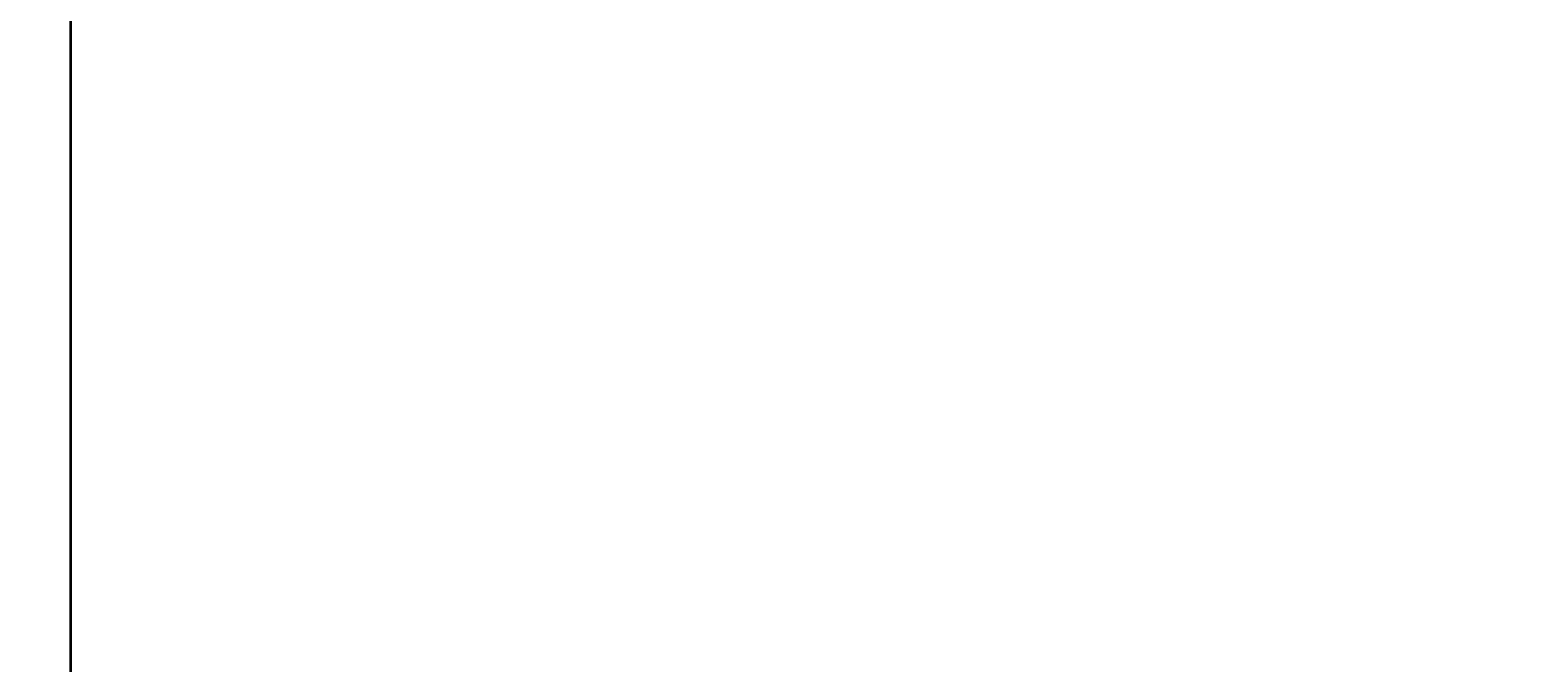
# Model space of a CAD drawing. Units: inches. Extents: x 2163 to 2982, y 1024 to 2288.
# Tile 12 of 22: x 2448 to 2532, y 1885 to 1920. Entities that reach past the tile are written whole.
import ezdxf

# ---------------------------------------------------------------- set-up
doc = ezdxf.new("R2010")
doc.units = ezdxf.units.IN
doc.layers.add('A-ANNO-DIMS', color=2, linetype='Continuous', lineweight=18)
doc.layers.add('A-WALL', color=7, linetype='Continuous', lineweight=35)
doc.styles.get("Standard").update_dxf_attribs({"font": 'arial.ttf'})
doc.dimstyles.get("Standard").update_dxf_attribs({"dimtxt": 0.18, "dimasz": 0.18, "dimexe": 0.18, "dimexo": 0.0625, "dimgap": 0.09, "dimtad": 0, "dimtih": 1, "dimtoh": 1, "dimdec": 4, "dimzin": 0, "dimdsep": 46, "dimtxsty": 'Standard', "dimcen": 0.09, "dimadec": 0, "dimazin": 0, "dimtfac": 1, "dimtdec": 4, "dimtofl": 0, "dimtmove": 0, "dimatfit": 3, "dimfxl": 1, "dimtolj": 1, "dimtzin": 0, "dimarcsym": 0})

# ---------------------------------------------------------------- blocks, each defined once
blk = doc.blocks.new('*D29')
at = {"layer": 'A-ANNO-DIMS', "color": 0, "lineweight": -2, "transparency": 16777216}
for p, q in [((2285.339, 1738.831), (2285.339, 2288.099)), ((2285.519, 2287.919), (2576.051, 2287.919)), ((2867.159, 2287.919), (2576.627, 2287.919)), ((2867.339, 2229.331), (2867.339, 2288.099))]:
    blk.add_line(p, q, dxfattribs=at)
at = {"layer": 'A-ANNO-DIMS', "color": 0, "transparency": 16777216}
for points in [[(2285.519, 2287.949), (2285.519, 2287.889), (2285.339, 2287.919)], [(2867.159, 2287.949), (2867.159, 2287.889), (2867.339, 2287.919)]]:
    blk.add_solid(points, dxfattribs=at)
at = {"layer": 'Defpoints', "color": 0, "transparency": 16777216}
for p in [(2867.339, 2287.919), (2867.339, 2229.269), (2285.339, 1738.769)]:
    blk.add_point(p, dxfattribs=at)
at = {"layer": 'A-ANNO-DIMS', "color": 0, "transparency": 16777216, "insert": (2576.339, 2287.919), "char_height": 0.18, "attachment_point": 5}
blk.add_mtext('\\A1;582', dxfattribs=at)

msp = doc.modelspace()

# ---------------------------------------------------------------- linework, layer by layer
at = {"layer": 'A-WALL'}
msp.add_line((2450.3389, 1963.7688), (2450.3389, 1879.973), dxfattribs=at)

# ---------------------------------------------------------------- dimensions: what is measured, and where the dimension line sits
at = {"layer": 'A-ANNO-DIMS'}
dim = msp.add_linear_dim(base=(2867.3389, 2287.9188), p1=(2285.3389, 1738.7688), p2=(2867.3389, 2229.2688), dimstyle='Standard', override={"dimdec": 0, "dimlfac": 1, "dimrnd": 0, "dimzin": 0, "dimdsep": 46, "dimlunit": 2}, dxfattribs=at)
dim.commit()
dim.dimension.update_dxf_attribs({"geometry": '*D29', "text_midpoint": (2576.3389, 2287.9188)})

doc.saveas('drawing.dxf')
